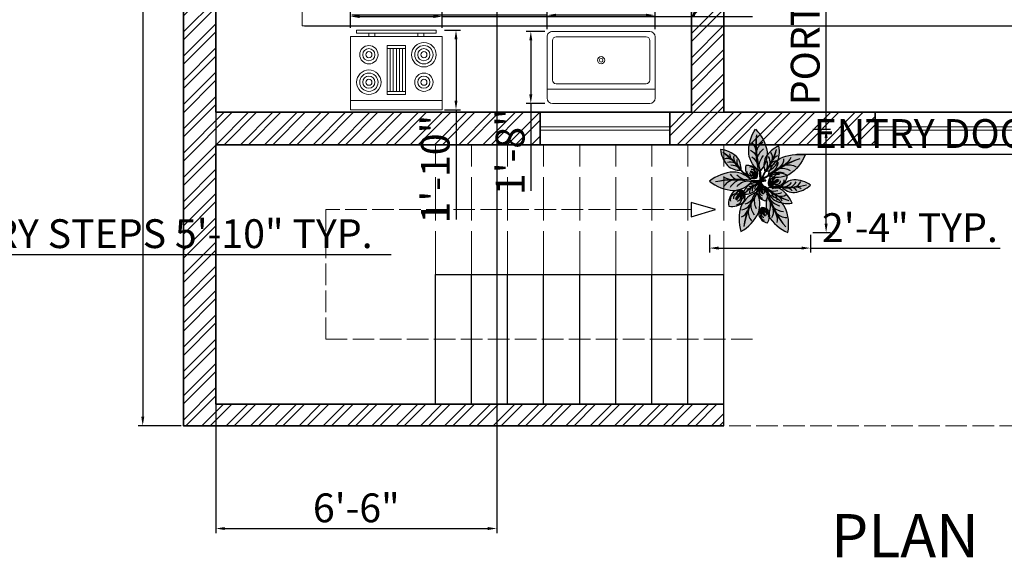
# Model space of a CAD drawing. Units: inches. Extents: x 3595 to 4516, y 2363 to 2965.
# Tile 6 of 12: x 4036 to 4309, y 2363 to 2512. Entities that reach past the tile are written whole.
import ezdxf

# ---------------------------------------------------------------- set-up
doc = ezdxf.new("R2010")
doc.units = ezdxf.units.IN
doc.linetypes.add('ACAD_ISO02W100', pattern=[15, 12, -3])
for name, color, linetype, lineweight in [('A-ANNO-DIMS', 2, 'Continuous', 18), ('A-ANNO-TEXT', 7, 'Continuous', 25), ('A-EQPM', 8, 'Continuous', 18), ('A-FLOR-CASE', 9, 'Continuous', 18), ('A-FLOR-FIXT', 8, 'Continuous', 18), ('A-FLOR-OTLN', 7, 'ACAD_ISO02W100', 18), ('A-FLOR-STRS', 7, 'Continuous', 25), ('A-FLOR-STRS-OVHD', 7, 'ACAD_ISO02W100', 18), ('A-GLAZ', 4, 'Continuous', 18), ('A-WALL', 7, 'Continuous', 35), ('L-PLNT', 3, 'Continuous', 13)]:
    doc.layers.add(name, color=color, linetype=linetype, lineweight=lineweight)
doc.layers.add('A-WALL-PATT', color=251, linetype='Continuous', lineweight=13, true_color=0x636466)
doc.layers.add('MESA', color=7, linetype='Continuous')
doc.styles.get("Standard").update_dxf_attribs({"font": 'arial.ttf'})
doc.dimstyles.new('ISO-25', dxfattribs={"dimtxt": 8, "dimasz": 2.5, "dimexe": 1.25, "dimexo": 0.625, "dimtad": 1, "dimdec": 1, "dimlunit": 3, "dimtxsty": 'Standard', "dimcen": 2.5, "dimadec": 0, "dimazin": 0, "dimtfac": 1, "dimtdec": 1, "dimtmove": 0, "dimatfit": 3, "dimfxl": 1, "dimarcsym": 0})

# ---------------------------------------------------------------- blocks, each defined once
blk = doc.blocks.new('*D6')
at = {"layer": 'A-ANNO-DIMS', "color": 0, "lineweight": -2, "transparency": 16777216}
for p, q in [((4080.62, 2903.04), (4068.71, 2903.04)), ((4069.96, 2900.54), (4069.96, 2401.54)), ((4080.62, 2399.04), (4068.71, 2399.04))]:
    blk.add_line(p, q, dxfattribs=at)
at = {"layer": 'A-ANNO-DIMS', "color": 0, "transparency": 16777216}
for points in [[(4069.55, 2900.54), (4070.38, 2900.54), (4069.96, 2903.04)], [(4069.55, 2401.54), (4070.38, 2401.54), (4069.96, 2399.04)]]:
    blk.add_solid(points, dxfattribs=at)
at = {"layer": 'Defpoints', "color": 0, "transparency": 16777216}
for p in [(4081.24, 2903.04), (4069.96, 2399.04), (4081.24, 2399.04)]:
    blk.add_point(p, dxfattribs=at)
at = {"layer": 'A-ANNO-DIMS', "color": 0, "transparency": 16777216, "insert": (4065.32, 2651.04), "char_height": 8, "attachment_point": 5, "rotation": 90}
blk.add_mtext("42'", dxfattribs=at)
blk = doc.blocks.new('folha Ant')
at = {"layer": 'MESA', "ltscale": 0.8}
h = blk.add_hatch(color=256, dxfattribs=at)
h.dxf.hatch_style = 1
h.set_gradient(color1=(179, 116, 77), color2=(114, 74, 49), one_color=1, tint=0.32, name='CURVED')
h.paths.add_polyline_path([(0.05, -0.0003), (0.0485, 0.0057, 0.033108), (0, 0, 0.809082), (0.002, -0.006, -0.032777)])
h.paths.add_polyline_path([(0.0973, 0.0049, 0.033108), (0.0485, 0.0057), (0.05, -0.0003, -0.032777), (0.0983, -0.001), (0.0953, 0.0026)])
h = blk.add_hatch(color=256, dxfattribs=at)
h.dxf.hatch_style = 1
h.set_gradient(color1=(103, 159, 96), color2=(52, 80, 48), one_color=1, tint=0.25)
h.paths.add_polyline_path([(0.3533, 0.0075, -0.09675), (0.0989, 0.0067, 0.007527), (0.0953, 0.0026, 0.014292), (0.1023, -0.0053, 0.086654)])
h = blk.add_hatch(color=256, dxfattribs=at)
h.dxf.hatch_style = 1
h.set_gradient(color1=(103, 159, 96), color2=(179, 207, 175), one_color=1, tint=0.75, name='INVCURVED')
h.paths.add_polyline_path([(0.2266, 0.0676, 0.199512), (0.0989, 0.0067, 0.09675), (0.3533, 0.0075, -0.086654), (0.1023, -0.0053, 0.192489), (0.2266, -0.0624, 0.158608), (0.3953, 0.0026, 0.158608)])
blk.add_lwpolyline([(0.0983, -0.001), (0.0953, 0.0026), (0.0973, 0.0049, 0.066288), (0, 0, 0.809082), (0.002, -0.006, -0.065625)], format="xyb", close=True, dxfattribs=at)
for centre, radius, start, end in [((0.2359, -0.1164), 0.1842, 92.91214, 139.76953), ((0.2359, 0.1215), 0.1842, 220.23047, 267.08786), ((0.2242, 0.6583), 0.6635, 259.11898, 281.22354), ((0.1912, 0.7199), 0.7306, 263.00966, 282.81986), ((0.1144, 0.1192), 0.1187, 277.64114, 318.48201), ((0.1515, 0.1013), 0.1129, 290.56342, 330.45391), ((0.211, -0.2242), 0.2922, 50.90546, 86.95539), ((0.211, 0.2293), 0.2922, 273.04461, 309.09454), ((0.2123, 0.0879), 0.0955, 283.00127, 333.19107), ((0.1127, -0.1239), 0.1214, 41.75279, 70.10606), ((0.1853, -0.0821), 0.0727, 27.73756, 79.23475), ((0.2381, -0.0995), 0.0902, 48.80268, 88.01103)]:
    blk.add_arc(centre, radius, start, end, dxfattribs=at)
blk = doc.blocks.new('folha A')
at = {"layer": 'MESA', "ltscale": 0.8}
h = blk.add_hatch(color=256, dxfattribs=at)
h.dxf.hatch_style = 1
h.set_gradient(color1=(237, 238, 238), one_color=1, tint=1)
h.paths.add_polyline_path([(0.15, 0, 0.256909), (0.0543, 0.05, 0.240303), (0.0028, 0.0075, -0.358381), (0.0489, 0.0306, 0.270233), (0, 0, -0.348977), (0.0363, 0.0149, 0.25095), (0.0039, 0, -0.245389), (0.0298, 0.008, 0.153246), (0.0082, 0, 0.15184), (0.0296, -0.008, 0.001374), (0.0298, -0.008, -0.245389), (0.0039, 0, 0.25095), (0.0363, -0.0149, -0.348977), (0, 0, 0.270233), (0.0489, -0.0306, -0.358381), (0.0028, -0.0075, 0.240303), (0.0543, -0.05, 0.256909)])
edge = h.paths.add_edge_path(flags=16)
edge.add_arc((0.0098, 0.0552), 0.0552, 269.91603, 271.41539, ccw=False)
edge.add_arc((0.011, -0.0487), 0.0487, 89.81625, 91.51517, ccw=False)
edge.add_arc((0.0098, 0.0552), 0.0552, 271.41539, 288.97446)
edge.add_spline(control_points=[(0.0278, 0.003), (0.0281, 0.003), (0.03, 0.0028), (0.032, 0.0025), (0.0337, 0.0022)], knot_values=[0.247151, 0.247151, 0.247151, 0.247151, 0.247786, 0.253074, 0.253074, 0.253074, 0.253074], degree=3, periodic=0)
edge.add_spline(control_points=[(0.0337, 0.0022), (0.0349, 0.0021), (0.0361, 0.0019), (0.0372, 0.0017)], knot_values=[0.243636, 0.243636, 0.243636, 0.243636, 0.247151, 0.247151, 0.247151, 0.247151], degree=3, periodic=0)
edge.add_spline(control_points=[(0.0372, 0.0017), (0.0385, 0.0015), (0.0405, 0.0013), (0.0424, 0.0011), (0.0431, 0.0011)], knot_values=[0.23773, 0.23773, 0.23773, 0.23773, 0.241748, 0.243636, 0.243636, 0.243636, 0.243636], degree=3, periodic=0)
edge.add_spline(control_points=[(0.0431, 0.0011), (0.044, 0.001), (0.045, 0.001), (0.0459, 0.001)], knot_values=[0.234818, 0.234818, 0.234818, 0.234818, 0.23773, 0.23773, 0.23773, 0.23773], degree=3, periodic=0)
edge.add_spline(control_points=[(0.0459, 0.001), (0.0472, 0.0009), (0.0485, 0.0009), (0.0498, 0.0009)], knot_values=[0.230931, 0.230931, 0.230931, 0.230931, 0.234818, 0.234818, 0.234818, 0.234818], degree=3, periodic=0)
edge.add_spline(control_points=[(0.0498, 0.0009), (0.0513, 0.0009), (0.0528, 0.0009), (0.0543, 0.0009)], knot_values=[0.226471, 0.226471, 0.226471, 0.226471, 0.230931, 0.230931, 0.230931, 0.230931], degree=3, periodic=0)
edge.add_spline(control_points=[(0.0543, 0.0009), (0.0547, 0.0009), (0.0564, 0.001), (0.0581, 0.001), (0.0594, 0.0011)], knot_values=[0.221526, 0.221526, 0.221526, 0.221526, 0.222579, 0.226471, 0.226471, 0.226471, 0.226471], degree=3, periodic=0)
edge.add_spline(control_points=[(0.0594, 0.0011), (0.0609, 0.0012), (0.0623, 0.0014), (0.0637, 0.0017)], knot_values=[0.217168, 0.217168, 0.217168, 0.217168, 0.221526, 0.221526, 0.221526, 0.221526], degree=3, periodic=0)
edge.add_spline(control_points=[(0.0637, 0.0017), (0.0648, 0.002), (0.066, 0.0024), (0.0672, 0.0029), (0.0674, 0.003)], knot_values=[0.213164, 0.213164, 0.213164, 0.213164, 0.216463, 0.217168, 0.217168, 0.217168, 0.217168], degree=3, periodic=0)
edge.add_spline(control_points=[(0.0674, 0.003), (0.0685, 0.0035), (0.07, 0.0044), (0.0718, 0.0051), (0.0724, 0.0052)], knot_values=[0.207777, 0.207777, 0.207777, 0.207777, 0.211372, 0.213164, 0.213164, 0.213164, 0.213164], degree=3, periodic=0)
edge.add_spline(control_points=[(0.0724, 0.0052), (0.0729, 0.0053), (0.0744, 0.0054), (0.0757, 0.0044), (0.0762, 0.0036)], knot_values=[0.203445, 0.203445, 0.203445, 0.203445, 0.204995, 0.207777, 0.207777, 0.207777, 0.207777], degree=3, periodic=0)
edge.add_spline(control_points=[(0.0762, 0.0036), (0.0763, 0.0036), (0.0768, 0.0026), (0.0767, 0.0012), (0.0763, 0), (0.0763, -0.0001)], knot_values=[0.199694, 0.199694, 0.199694, 0.199694, 0.199863, 0.203137, 0.203445, 0.203445, 0.203445, 0.203445], degree=3, periodic=0)
edge.add_spline(control_points=[(0.0763, -0.0001), (0.0761, -0.0008), (0.0757, -0.0017), (0.075, -0.0024), (0.0748, -0.0026)], knot_values=[0.196756, 0.196756, 0.196756, 0.196756, 0.198903, 0.199694, 0.199694, 0.199694, 0.199694], degree=3, periodic=0)
edge.add_spline(control_points=[(0.0748, -0.0026), (0.0743, -0.0031), (0.0734, -0.0037), (0.0725, -0.0042), (0.0722, -0.0043)], knot_values=[0.193643, 0.193643, 0.193643, 0.193643, 0.195869, 0.196756, 0.196756, 0.196756, 0.196756], degree=3, periodic=0)
edge.add_spline(control_points=[(0.0722, -0.0043), (0.0708, -0.0049), (0.0694, -0.0052), (0.0678, -0.0054)], knot_values=[0.189135, 0.189135, 0.189135, 0.189135, 0.193643, 0.193643, 0.193643, 0.193643], degree=3, periodic=0)
edge.add_spline(control_points=[(0.0678, -0.0054), (0.0677, -0.0054), (0.0667, -0.0056), (0.0657, -0.0057), (0.0648, -0.0058)], knot_values=[0.186092, 0.186092, 0.186092, 0.186092, 0.186502, 0.189135, 0.189135, 0.189135, 0.189135], degree=3, periodic=0)
edge.add_spline(control_points=[(0.0648, -0.0058), (0.0635, -0.0059), (0.0621, -0.006), (0.0608, -0.0061)], knot_values=[0.182083, 0.182083, 0.182083, 0.182083, 0.186092, 0.186092, 0.186092, 0.186092], degree=3, periodic=0)
edge.add_spline(control_points=[(0.0608, -0.0061), (0.0596, -0.0062), (0.0584, -0.0062), (0.0571, -0.0062)], knot_values=[0.178391, 0.178391, 0.178391, 0.178391, 0.182083, 0.182083, 0.182083, 0.182083], degree=3, periodic=0)
edge.add_spline(control_points=[(0.0571, -0.0062), (0.0568, -0.0062), (0.0555, -0.0063), (0.0543, -0.0063), (0.0534, -0.0063)], knot_values=[0.17468, 0.17468, 0.17468, 0.17468, 0.175797, 0.178391, 0.178391, 0.178391, 0.178391], degree=3, periodic=0)
edge.add_spline(control_points=[(0.0534, -0.0063), (0.0525, -0.0063), (0.0516, -0.0063), (0.0506, -0.0063)], knot_values=[0.171864, 0.171864, 0.171864, 0.171864, 0.17468, 0.17468, 0.17468, 0.17468], degree=3, periodic=0)
edge.add_spline(control_points=[(0.0506, -0.0063), (0.0494, -0.0063), (0.0482, -0.0063), (0.047, -0.0062)], knot_values=[0.16826, 0.16826, 0.16826, 0.16826, 0.171864, 0.171864, 0.171864, 0.171864], degree=3, periodic=0)
edge.add_spline(control_points=[(0.047, -0.0062), (0.0453, -0.0061), (0.0434, -0.006), (0.0414, -0.0057), (0.0411, -0.0057)], knot_values=[0.162342, 0.162342, 0.162342, 0.162342, 0.167388, 0.16826, 0.16826, 0.16826, 0.16826], degree=3, periodic=0)
edge.add_spline(control_points=[(0.0411, -0.0057), (0.0399, -0.0055), (0.0386, -0.0053), (0.0374, -0.005)], knot_values=[0.158654, 0.158654, 0.158654, 0.158654, 0.162342, 0.162342, 0.162342, 0.162342], degree=3, periodic=0)
edge.add_spline(control_points=[(0.0374, -0.005), (0.0365, -0.0049), (0.0357, -0.0047), (0.0348, -0.0045)], knot_values=[0.156033, 0.156033, 0.156033, 0.156033, 0.158654, 0.158654, 0.158654, 0.158654], degree=3, periodic=0)
edge.add_spline(control_points=[(0.0348, -0.0045), (0.0335, -0.0043), (0.0317, -0.004), (0.03, -0.0037), (0.0295, -0.0036)], knot_values=[0.15048, 0.15048, 0.15048, 0.15048, 0.154549, 0.156033, 0.156033, 0.156033, 0.156033], degree=3, periodic=0)
edge.add_arc((0.011, -0.0487), 0.0487, 67.70537, 89.81625)
h = blk.add_hatch(color=256, dxfattribs=at)
h.dxf.hatch_style = 1
h.set_gradient(color1=(117, 211, 105), one_color=1, tint=1)
h.paths.add_polyline_path([(0.0489, 0.0306, 0.358381), (0.0028, 0.0075, 0.02724), (0, 0, -0.270233)])
h.paths.add_polyline_path([(0.0039, 0, -0.25095), (0.0363, 0.0149, 0.348977), (0, 0, 0.348977), (0.0363, -0.0149, -0.25095)])
h.paths.add_polyline_path([(0.0298, 0.008, 0.245389), (0.0039, 0, 0.245389), (0.0298, -0.008, -0.153246), (0.0082, 0, -0.153246)], flags=17)
h.paths.add_polyline_path([(0, 0, 0.02724), (0.0028, -0.0075, 0.358381), (0.0489, -0.0306, -0.270233)])
h = blk.add_hatch(color=256, dxfattribs=at)
h.dxf.hatch_style = 1
h.set_gradient(color1=(68, 182, 53), color2=(121, 213, 109), one_color=1, tint=0.63, name='CYLINDER')
edge = h.paths.add_edge_path()
edge.add_spline(control_points=[(0.0722, -0.0043), (0.0725, -0.0042), (0.0734, -0.0037), (0.0743, -0.0031), (0.0748, -0.0026)], knot_values=[0.193643, 0.193643, 0.193643, 0.193643, 0.194531, 0.196756, 0.196756, 0.196756, 0.196756], degree=3, periodic=0)
edge.add_spline(control_points=[(0.0748, -0.0026), (0.075, -0.0024), (0.0757, -0.0017), (0.0761, -0.0008), (0.0763, -0.0001)], knot_values=[0.196756, 0.196756, 0.196756, 0.196756, 0.197548, 0.199694, 0.199694, 0.199694, 0.199694], degree=3, periodic=0)
edge.add_spline(control_points=[(0.0763, -0.0001), (0.0763, 0), (0.0767, 0.0012), (0.0768, 0.0026), (0.0763, 0.0036), (0.0762, 0.0036)], knot_values=[0.199694, 0.199694, 0.199694, 0.199694, 0.200002, 0.203276, 0.203445, 0.203445, 0.203445, 0.203445], degree=3, periodic=0)
edge.add_spline(control_points=[(0.0762, 0.0036), (0.0757, 0.0044), (0.0744, 0.0054), (0.0729, 0.0053), (0.0724, 0.0052)], knot_values=[0.203445, 0.203445, 0.203445, 0.203445, 0.206228, 0.207777, 0.207777, 0.207777, 0.207777], degree=3, periodic=0)
edge.add_spline(control_points=[(0.0724, 0.0052), (0.0718, 0.0051), (0.07, 0.0044), (0.0685, 0.0035), (0.0674, 0.003)], knot_values=[0.207777, 0.207777, 0.207777, 0.207777, 0.20957, 0.213164, 0.213164, 0.213164, 0.213164], degree=3, periodic=0)
edge.add_spline(control_points=[(0.0674, 0.003), (0.0672, 0.0029), (0.066, 0.0024), (0.0648, 0.002), (0.0637, 0.0017)], knot_values=[0.213164, 0.213164, 0.213164, 0.213164, 0.213868, 0.217168, 0.217168, 0.217168, 0.217168], degree=3, periodic=0)
edge.add_spline(control_points=[(0.0637, 0.0017), (0.0623, 0.0014), (0.0609, 0.0012), (0.0594, 0.0011)], knot_values=[0.217168, 0.217168, 0.217168, 0.217168, 0.221526, 0.221526, 0.221526, 0.221526], degree=3, periodic=0)
edge.add_spline(control_points=[(0.0594, 0.0011), (0.0581, 0.001), (0.0564, 0.001), (0.0547, 0.0009), (0.0543, 0.0009)], knot_values=[0.221526, 0.221526, 0.221526, 0.221526, 0.225418, 0.226471, 0.226471, 0.226471, 0.226471], degree=3, periodic=0)
edge.add_spline(control_points=[(0.0543, 0.0009), (0.0528, 0.0009), (0.0513, 0.0009), (0.0498, 0.0009)], knot_values=[0.226471, 0.226471, 0.226471, 0.226471, 0.230931, 0.230931, 0.230931, 0.230931], degree=3, periodic=0)
edge.add_spline(control_points=[(0.0498, 0.0009), (0.0485, 0.0009), (0.0472, 0.0009), (0.0459, 0.001)], knot_values=[0.230931, 0.230931, 0.230931, 0.230931, 0.234818, 0.234818, 0.234818, 0.234818], degree=3, periodic=0)
edge.add_spline(control_points=[(0.0459, 0.001), (0.045, 0.001), (0.044, 0.001), (0.0431, 0.0011)], knot_values=[0.234818, 0.234818, 0.234818, 0.234818, 0.23773, 0.23773, 0.23773, 0.23773], degree=3, periodic=0)
edge.add_spline(control_points=[(0.0431, 0.0011), (0.0424, 0.0011), (0.0405, 0.0013), (0.0385, 0.0015), (0.0372, 0.0017)], knot_values=[0.23773, 0.23773, 0.23773, 0.23773, 0.239619, 0.243636, 0.243636, 0.243636, 0.243636], degree=3, periodic=0)
edge.add_spline(control_points=[(0.0372, 0.0017), (0.0361, 0.0019), (0.0349, 0.0021), (0.0337, 0.0022)], knot_values=[0.243636, 0.243636, 0.243636, 0.243636, 0.247151, 0.247151, 0.247151, 0.247151], degree=3, periodic=0)
edge.add_spline(control_points=[(0.0337, 0.0022), (0.032, 0.0025), (0.03, 0.0028), (0.0281, 0.003), (0.0278, 0.003)], knot_values=[0.247151, 0.247151, 0.247151, 0.247151, 0.25244, 0.253074, 0.253074, 0.253074, 0.253074], degree=3, periodic=0)
edge.add_arc((0.011, 0.0487), 0.0487, 271.51517, 290.22735, ccw=False)
edge.add_arc((0.011, -0.0487), 0.0487, 67.70537, 88.48483, ccw=False)
edge.add_spline(control_points=[(0.0295, -0.0036), (0.03, -0.0037), (0.0317, -0.004), (0.0335, -0.0043), (0.0348, -0.0045)], knot_values=[0.15048, 0.15048, 0.15048, 0.15048, 0.151964, 0.156033, 0.156033, 0.156033, 0.156033], degree=3, periodic=0)
edge.add_spline(control_points=[(0.0348, -0.0045), (0.0357, -0.0047), (0.0365, -0.0049), (0.0374, -0.005)], knot_values=[0.156033, 0.156033, 0.156033, 0.156033, 0.158654, 0.158654, 0.158654, 0.158654], degree=3, periodic=0)
edge.add_spline(control_points=[(0.0374, -0.005), (0.0386, -0.0053), (0.0399, -0.0055), (0.0411, -0.0057)], knot_values=[0.158654, 0.158654, 0.158654, 0.158654, 0.162342, 0.162342, 0.162342, 0.162342], degree=3, periodic=0)
edge.add_spline(control_points=[(0.0411, -0.0057), (0.0414, -0.0057), (0.0434, -0.006), (0.0453, -0.0061), (0.047, -0.0062)], knot_values=[0.162342, 0.162342, 0.162342, 0.162342, 0.163214, 0.16826, 0.16826, 0.16826, 0.16826], degree=3, periodic=0)
edge.add_spline(control_points=[(0.047, -0.0062), (0.0482, -0.0063), (0.0494, -0.0063), (0.0506, -0.0063)], knot_values=[0.16826, 0.16826, 0.16826, 0.16826, 0.171864, 0.171864, 0.171864, 0.171864], degree=3, periodic=0)
edge.add_spline(control_points=[(0.0506, -0.0063), (0.0516, -0.0063), (0.0525, -0.0063), (0.0534, -0.0063)], knot_values=[0.171864, 0.171864, 0.171864, 0.171864, 0.17468, 0.17468, 0.17468, 0.17468], degree=3, periodic=0)
edge.add_spline(control_points=[(0.0534, -0.0063), (0.0543, -0.0063), (0.0555, -0.0063), (0.0568, -0.0062), (0.0571, -0.0062)], knot_values=[0.17468, 0.17468, 0.17468, 0.17468, 0.177274, 0.178391, 0.178391, 0.178391, 0.178391], degree=3, periodic=0)
edge.add_spline(control_points=[(0.0571, -0.0062), (0.0584, -0.0062), (0.0596, -0.0062), (0.0608, -0.0061)], knot_values=[0.178391, 0.178391, 0.178391, 0.178391, 0.182083, 0.182083, 0.182083, 0.182083], degree=3, periodic=0)
edge.add_spline(control_points=[(0.0608, -0.0061), (0.0621, -0.006), (0.0635, -0.0059), (0.0648, -0.0058)], knot_values=[0.182083, 0.182083, 0.182083, 0.182083, 0.186092, 0.186092, 0.186092, 0.186092], degree=3, periodic=0)
edge.add_spline(control_points=[(0.0648, -0.0058), (0.0657, -0.0057), (0.0667, -0.0056), (0.0677, -0.0054), (0.0678, -0.0054)], knot_values=[0.186092, 0.186092, 0.186092, 0.186092, 0.188726, 0.189135, 0.189135, 0.189135, 0.189135], degree=3, periodic=0)
edge.add_spline(control_points=[(0.0678, -0.0054), (0.0694, -0.0052), (0.0708, -0.0049), (0.0722, -0.0043)], knot_values=[0.189135, 0.189135, 0.189135, 0.189135, 0.193643, 0.193643, 0.193643, 0.193643], degree=3, periodic=0)
for p, q in [((0.0299, -0.0008), (0.0236, 0.0003)), ((0.0324, 0.0004), (0.0358, 0.0051)), ((0.0367, 0.001), (0.0414, 0.0073)), ((0.0435, -0.0027), (0.0427, 0.0041)), ((0.0455, -0.0007), (0.0466, 0.0032)), ((0.0507, -0.0021), (0.0477, 0.0086)), ((0.0545, -0.0006), (0.0538, 0.005)), ((0.0604, -0.0013), (0.0571, 0.0065)), ((0.0637, -0.0003), (0.0638, 0.0057)), ((0.0674, 0.0003), (0.0674, 0.0088)), ((0.071, 0.0011), (0.0736, 0.0087)), ((0.0744, 0.0005), (0.0836, -0.0024)), ((0.0745, 0.0023), (0.0809, 0.0072)), ((0.0331, -0.0017), (0.0356, -0.0058)), ((0.0359, -0.0021), (0.0384, -0.0071)), ((0.04, -0.0018), (0.0423, -0.0098)), ((0.0474, -0.0047), (0.0459, -0.0105)), ((0.0512, -0.005), (0.0493, -0.009)), ((0.0546, -0.0037), (0.0519, -0.0097)), ((0.0571, -0.0045), (0.0573, -0.0126)), ((0.0629, -0.0036), (0.0579, -0.0096)), ((0.0649, -0.0044), (0.0646, -0.0097)), ((0.0679, -0.003), (0.0676, -0.0121)), ((0.0718, -0.0029), (0.0733, -0.0082)), ((0.0731, -0.0013), (0.0781, -0.005))]:
    blk.add_line(p, q, dxfattribs=at)
for centre, radius, start, end in [((0.0702, -0.0218), 0.0735, 102.48764, 162.77768), ((0.0507, -0.0267), 0.0573, 91.76636, 152.2545), ((0.0275, -0.0154), 0.0315, 73.89832, 150.84957), ((0.0399, -0.009), 0.0406, 77.14264, 158.36501), ((0.034, -0.0228), 0.0378, 86.58524, 142.93515), ((0.0245, -0.0208), 0.0293, 79.57473, 134.72404), ((0.0317, -0.0305), 0.0385, 92.86525, 127.71548), ((0.0067, 0.0482), 0.0483, 273.5313, 328.711), ((0.0098, 0.0552), 0.0552, 269.91603, 311.56133), ((0.011, -0.0487), 0.0487, 43.37027, 91.51517), ((0.0655, -0.0023), 0.025, 51.97118, 139.68499), ((0.0788, 0.0012), 0.0378, 48.94459, 144.53335), ((0.0567, -0.062), 0.112, 33.59498, 91.22784), ((0.0507, 0.0267), 0.0573, 207.7455, 268.23364), ((0.0275, 0.0154), 0.0315, 209.15043, 286.10168), ((0.0702, 0.0218), 0.0735, 197.22232, 257.51236), ((0.0399, 0.009), 0.0406, 201.63499, 282.85736), ((0.034, 0.0228), 0.0378, 217.06485, 273.41476), ((0.0245, 0.0208), 0.0293, 225.27596, 280.42527), ((0.0317, 0.0305), 0.0385, 232.28452, 267.13475), ((0.0067, -0.0482), 0.0483, 31.289, 86.4687), ((0.0676, -0.0011), 0.0254, 213.67702, 332.84146), ((0.0804, 0.0017), 0.0409, 217.4348, 331.73221), ((0.0567, 0.062), 0.112, 268.77216, 326.40502)]:
    blk.add_arc(centre, radius, start, end, dxfattribs=at)
blk.add_open_spline([(0.0295, -0.0036), (0.03, -0.0037), (0.0339, -0.0043), (0.0429, -0.0064), (0.0552, -0.0064), (0.0655, -0.0059), (0.0723, -0.0047), (0.0754, -0.0023), (0.0766, 0.0004), (0.0769, 0.0036), (0.0738, 0.0058), (0.0702, 0.0046), (0.0648, 0.0013), (0.0544, 0.0009), (0.0416, 0.0008), (0.0325, 0.0025), (0.0281, 0.003), (0.0278, 0.003)], degree=3, knots=[0.1504802, 0.1504802, 0.1504802, 0.1504802, 0.1519644, 0.163214, 0.177274, 0.1887256, 0.1945307, 0.1975476, 0.2000024, 0.2032763, 0.2062279, 0.2095699, 0.2138685, 0.2254176, 0.2396186, 0.2524399, 0.2530743, 0.2530743, 0.2530743, 0.2530743], dxfattribs=at)
blk = doc.blocks.new('Anturio Completa')
at = {"layer": 'MESA', "xscale": -1}
for p, rotation in [((0.0382, -0.3934), 275.9103487005753), ((0.0047, -0.3743), 209.3422747969654)]:
    blk.add_blockref('folha Ant', p, dxfattribs=dict(at, rotation=rotation))
at = {"layer": 'MESA'}
for name, p, xscale, yscale, zscale, rotation in [('folha Ant', (-0.0545, -0.3355), 0.6875195991113106, 0.6875195991113106, 0.6875195991113106, 134.6123703789177), ('folha Ant', (0.0396, -0.3604), 0.6875195991112988, 0.6875195991112988, 0.6875195991112988, 62.02852832027476), ('folha A', (0.0091, -0.3436), 0.7678141644548924, 0.7678141644548924, 0.7678141644548924, 132.2423739965673), ('folha Ant', (0.06, -0.3566), 0.4588451896756128, 0.4588451896756128, 0.4588451896756128, 214.0760858842101), ('folha Ant', (0.0225, -0.3869), 0.6875195991113232, 0.6875195991113232, 0.6875195991113232, 329.7037252995857), ('folha A', (0.0322, -0.3992), 0.7678141644548587, 0.7678141644548587, 0.7678141644548587, 290.0444626994612), ('folha Ant', (0.1178, -0.4144), 0.6875195991112375, 0.6875195991112375, 0.6875195991112375, 3.732606609119443), ('folha A', (0.0446, -0.5537), 0.7678141644548587, 0.7678141644548587, 0.7678141644548587, 290.0444626994612)]:
    blk.add_blockref(name, p, dxfattribs=dict(at, xscale=xscale, yscale=yscale, zscale=zscale, rotation=rotation))
for name, p, rotation in [('folha Ant', (0.0722, -0.3656), 180), ('folha Ant', (0.0428, -0.3558), 248.0349850699403), ('folha A', (0.0917, -0.3951), 27.20904127110871), ('folha A', (-0.0806, -0.4387), 224.8255080541778), ('folha Ant', (0.0423, -0.3813), 297.7195320534174)]:
    blk.add_blockref(name, p, dxfattribs=dict(at, rotation=rotation))
blk = doc.blocks.new('Range-Oven - 30 in top')
for p, q in [((0, -3), (30, -3)), ((12, -6), (18, -6)), ((13, -20), (13, -6)), ((14, -6), (14, -20)), ((15, -20), (15, -6)), ((16, -6), (16, -20)), ((17, -20), (17, -6)), ((18, -20), (12, -20)), ((6, -24), (6, -25)), ((8, -25), (8, -24)), ((22, -25), (22, -24)), ((24, -24), (24, -25))]:
    blk.add_line(p, q)
for points in [[(0, -24), (0, 0), (30, 0), (30, -24)], [(12, -21), (12, -5), (18, -5), (18, -21)], [(2, -26), (2, -25), (28, -25), (28, -26)]]:
    blk.add_lwpolyline(points, close=True)
for centre, radius in [((6, -9), 4), ((6, -9), 3), ((24, -9), 3), ((6, -9), 2), ((6, -9), 1), ((24, -9), 2), ((24, -9), 1), ((6, -18), 3), ((6, -18), 2), ((24, -18), 4), ((24, -18), 3), ((24, -18), 2), ((6, -18), 1), ((24, -18), 1)]:
    blk.add_circle(centre, radius)
blk = doc.blocks.new('Sink-single - 30 in top')
blk.add_line((-15, -3.999996), (15, -3.999996))
for points in [[(-13.5, 0), (13.5, 0)], [(-15, -18.499996), (-15, -1.5)], [(15, -1.5), (15, -18.499996)], [(-13.5, -17.499996), (-13.5, -6.499996)], [(-12.5, -5.499996), (12.5, -5.499996)], [(13.5, -6.499996), (13.5, -17.499996)], [(12.5, -18.499996), (-12.5, -18.499996)], [(13.5, -19.999996), (-13.5, -19.999996)]]:
    blk.add_lwpolyline(points)
for radius in [1, 0.5]:
    blk.add_circle((0, -11.999996), radius)
for centre, radius, start, end in [((-13.5, -1.5), 1.5, 90, 180), ((13.5, -1.5), 1.5, 0, 90), ((-12.5, -6.499996), 1, 90, 180), ((12.5, -6.499996), 1, 0, 90), ((-13.5, -18.499996), 1.5, 180, 270), ((-12.5, -17.499996), 1, 180, 270), ((12.5, -17.499996), 1, 270, 0), ((13.5, -18.499996), 1.5, 270, 0)]:
    blk.add_arc(centre, radius, start, end)
blk = doc.blocks.new('WIN-GLAZING-66IN')
for p, q in [((0, 1), (66, 1)), ((0, 0), (66, 0))]:
    blk.add_line(p, q)
blk = doc.blocks.new('WIN-GLAZING-36IN')
for p, q in [((0, 1), (36, 1)), ((0, 0), (36, 0))]:
    blk.add_line(p, q)
blk = doc.blocks.new('*D113')
at = {"layer": 'A-ANNO-DIMS', "color": 0, "lineweight": -2, "transparency": 16777216}
for p, q in [((4381.24, 2480.92), (4381.24, 2473.09)), ((4429.24, 2480.92), (4429.24, 2473.09)), ((4381.24, 2474.34), (4251.53, 2474.34)), ((4426.74, 2474.34), (4383.74, 2474.34))]:
    blk.add_line(p, q, dxfattribs=at)
at = {"layer": 'A-ANNO-DIMS', "color": 0, "transparency": 16777216}
for points in [[(4383.74, 2474.76), (4383.74, 2473.93), (4381.24, 2474.34)], [(4426.74, 2474.76), (4426.74, 2473.93), (4429.24, 2474.34)]]:
    blk.add_solid(points, dxfattribs=at)
at = {"layer": 'Defpoints', "color": 0, "transparency": 16777216}
for p in [(4381.24, 2481.54), (4429.24, 2481.54), (4381.24, 2474.34)]:
    blk.add_point(p, dxfattribs=at)
at = {"layer": 'A-ANNO-DIMS', "color": 0, "transparency": 16777216, "insert": (4315.14, 2479.11), "char_height": 8, "attachment_point": 5}
blk.add_mtext('ENTRY DOOR 4\'-0" TYP.', dxfattribs=at)
blk = doc.blocks.new('*D117')
at = {"layer": 'A-ANNO-DIMS', "color": 0, "lineweight": -2, "transparency": 16777216}
for p, q in [((3929.89, 2456.42), (3929.89, 2445.29)), ((3999.89, 2456.42), (3999.89, 2445.29)), ((3932.39, 2446.54), (3997.39, 2446.54)), ((3999.89, 2446.54), (4138.93, 2446.54))]:
    blk.add_line(p, q, dxfattribs=at)
at = {"layer": 'A-ANNO-DIMS', "color": 0, "transparency": 16777216}
for points in [[(3932.39, 2446.96), (3932.39, 2446.13), (3929.89, 2446.54)], [(3997.39, 2446.96), (3997.39, 2446.13), (3999.89, 2446.54)]]:
    blk.add_solid(points, dxfattribs=at)
at = {"layer": 'Defpoints', "color": 0, "transparency": 16777216}
for p in [(3929.89, 2457.04), (3999.89, 2457.04), (3999.89, 2446.54)]:
    blk.add_point(p, dxfattribs=at)
at = {"layer": 'A-ANNO-DIMS', "color": 0, "transparency": 16777216, "insert": (4070.66, 2451.31), "char_height": 8, "attachment_point": 5}
blk.add_mtext('ENTRY STEPS 5\'-10" TYP.', dxfattribs=at)
blk = doc.blocks.new('*D135')
at = {"layer": 'A-ANNO-DIMS', "color": 0, "lineweight": -2, "transparency": 16777216}
for p, q in [((4127.63, 2509.45), (4127.63, 2513.89)), ((4130.13, 2512.64), (4150.59, 2512.64)), ((4153.09, 2509.45), (4153.09, 2513.89)), ((4153.09, 2512.64), (4239.18, 2512.64))]:
    blk.add_line(p, q, dxfattribs=at)
at = {"layer": 'A-ANNO-DIMS', "color": 0, "transparency": 16777216}
for points in [[(4130.13, 2513.06), (4130.13, 2512.22), (4127.63, 2512.64)], [(4150.59, 2513.06), (4150.59, 2512.22), (4153.09, 2512.64)]]:
    blk.add_solid(points, dxfattribs=at)
at = {"layer": 'Defpoints', "color": 0, "transparency": 16777216}
for p in [(4153.09, 2512.64), (4127.63, 2508.82), (4153.09, 2508.82)]:
    blk.add_point(p, dxfattribs=at)
at = {"layer": 'A-ANNO-DIMS', "color": 0, "transparency": 16777216, "insert": (4197.38, 2517.4), "char_height": 8, "attachment_point": 5}
blk.add_mtext('RANGE 2\'-1 1/2"', dxfattribs=at)
blk = doc.blocks.new('*D136')
at = {"layer": 'A-ANNO-DIMS', "color": 0, "lineweight": -2, "transparency": 16777216}
for p, q in [((4153.71, 2508.82), (4158.16, 2508.82)), ((4156.91, 2506.32), (4156.91, 2489.26)), ((4153.71, 2486.76), (4158.16, 2486.76)), ((4156.91, 2486.76), (4156.91, 2456.28))]:
    blk.add_line(p, q, dxfattribs=at)
at = {"layer": 'A-ANNO-DIMS', "color": 0, "transparency": 16777216}
for points in [[(4156.49, 2506.32), (4157.32, 2506.32), (4156.91, 2508.82)], [(4156.49, 2489.26), (4157.32, 2489.26), (4156.91, 2486.76)]]:
    blk.add_solid(points, dxfattribs=at)
at = {"layer": 'Defpoints', "color": 0, "transparency": 16777216}
for p in [(4153.09, 2508.82), (4153.09, 2486.76), (4156.91, 2486.76)]:
    blk.add_point(p, dxfattribs=at)
at = {"layer": 'A-ANNO-DIMS', "color": 0, "transparency": 16777216, "insert": (4152.2, 2470.27), "char_height": 8, "attachment_point": 5, "rotation": 90}
blk.add_mtext('1\'-10"', dxfattribs=at)
blk = doc.blocks.new('*D137')
at = {"layer": 'A-ANNO-DIMS', "color": 0, "lineweight": -2, "transparency": 16777216}
for p, q in [((4182.18, 2512.99), (4128.01, 2512.99)), ((4182.18, 2509.12), (4182.18, 2514.24)), ((4209.68, 2512.99), (4184.68, 2512.99)), ((4212.18, 2509.12), (4212.18, 2514.24))]:
    blk.add_line(p, q, dxfattribs=at)
at = {"layer": 'A-ANNO-DIMS', "color": 0, "transparency": 16777216}
for points in [[(4184.68, 2513.41), (4184.68, 2512.58), (4182.18, 2512.99)], [(4209.68, 2513.41), (4209.68, 2512.58), (4212.18, 2512.99)]]:
    blk.add_solid(points, dxfattribs=at)
at = {"layer": 'Defpoints', "color": 0, "transparency": 16777216}
for p in [(4182.18, 2512.99), (4182.18, 2508.49), (4212.18, 2508.49)]:
    blk.add_point(p, dxfattribs=at)
at = {"layer": 'A-ANNO-DIMS', "color": 0, "transparency": 16777216, "insert": (4153.84, 2517.75), "char_height": 8, "attachment_point": 5}
blk.add_mtext('SINK 2\'-6"', dxfattribs=at)
blk = doc.blocks.new('*D138')
at = {"layer": 'A-ANNO-DIMS', "color": 0, "lineweight": -2, "transparency": 16777216}
for p, q in [((4181.55, 2508.49), (4176.43, 2508.49)), ((4177.68, 2505.99), (4177.68, 2490.99)), ((4181.55, 2488.49), (4176.43, 2488.49)), ((4177.68, 2488.49), (4177.68, 2464.23))]:
    blk.add_line(p, q, dxfattribs=at)
at = {"layer": 'A-ANNO-DIMS', "color": 0, "transparency": 16777216}
for points in [[(4177.26, 2505.99), (4178.09, 2505.99), (4177.68, 2508.49)], [(4177.26, 2490.99), (4178.09, 2490.99), (4177.68, 2488.49)]]:
    blk.add_solid(points, dxfattribs=at)
at = {"layer": 'Defpoints', "color": 0, "transparency": 16777216}
for p in [(4182.18, 2508.49), (4177.68, 2488.49), (4182.18, 2488.49)]:
    blk.add_point(p, dxfattribs=at)
at = {"layer": 'A-ANNO-DIMS', "color": 0, "transparency": 16777216, "insert": (4172.97, 2475.11), "char_height": 8, "attachment_point": 5, "rotation": 90}
blk.add_mtext('1\'-8"', dxfattribs=at)
blk = doc.blocks.new('*D145')
at = {"layer": 'A-ANNO-DIMS', "color": 0, "lineweight": -2, "transparency": 16777216}
for p, q in [((4259.64, 2481.4), (4259.64, 2645.3)), ((4255.95, 2481.4), (4260.89, 2481.4)), ((4259.64, 2455.16), (4259.64, 2478.9)), ((4255.95, 2452.66), (4260.89, 2452.66))]:
    blk.add_line(p, q, dxfattribs=at)
at = {"layer": 'A-ANNO-DIMS', "color": 0, "transparency": 16777216}
for points in [[(4259.22, 2478.9), (4260.06, 2478.9), (4259.64, 2481.4)], [(4259.22, 2455.16), (4260.06, 2455.16), (4259.64, 2452.66)]]:
    blk.add_solid(points, dxfattribs=at)
at = {"layer": 'Defpoints', "color": 0, "transparency": 16777216}
for p in [(4255.33, 2481.4), (4259.64, 2481.4), (4255.33, 2452.66)]:
    blk.add_point(p, dxfattribs=at)
at = {"layer": 'A-ANNO-DIMS', "color": 0, "transparency": 16777216, "insert": (4254.87, 2564.6), "char_height": 8, "attachment_point": 5, "rotation": 90}
blk.add_mtext('PORTICO PLANT 2\'-4 1/2" TYP.', dxfattribs=at)
blk = doc.blocks.new('*D146')
at = {"layer": 'A-ANNO-DIMS', "color": 0, "lineweight": -2, "transparency": 16777216}
for p, q in [((4227.3, 2452.03), (4227.3, 2447.1)), ((4255.33, 2452.03), (4255.33, 2447.1)), ((4229.8, 2448.35), (4252.83, 2448.35)), ((4255.33, 2448.35), (4307.98, 2448.35))]:
    blk.add_line(p, q, dxfattribs=at)
at = {"layer": 'A-ANNO-DIMS', "color": 0, "transparency": 16777216}
for points in [[(4229.8, 2448.77), (4229.8, 2447.93), (4227.3, 2448.35)], [(4252.83, 2448.77), (4252.83, 2447.93), (4255.33, 2448.35)]]:
    blk.add_solid(points, dxfattribs=at)
at = {"layer": 'Defpoints', "color": 0, "transparency": 16777216}
for p in [(4227.3, 2452.66), (4255.33, 2452.66), (4255.33, 2448.35)]:
    blk.add_point(p, dxfattribs=at)
at = {"layer": 'A-ANNO-DIMS', "color": 0, "transparency": 16777216, "insert": (4282.9, 2452.99), "char_height": 8, "attachment_point": 5}
blk.add_mtext('2\'-4" TYP.', dxfattribs=at)
blk = doc.blocks.new('*D160')
at = {"layer": 'A-ANNO-DIMS', "color": 0, "lineweight": -2, "transparency": 16777216}
for p, q in [((4114.87, 2510.04), (4471.04, 2510.04)), ((4469.79, 2488.54), (4469.79, 2507.54)), ((4090.87, 2486.04), (4471.04, 2486.04))]:
    blk.add_line(p, q, dxfattribs=at)
at = {"layer": 'A-ANNO-DIMS', "color": 0, "transparency": 16777216}
for points in [[(4469.38, 2507.54), (4470.21, 2507.54), (4469.79, 2510.04)], [(4469.38, 2488.54), (4470.21, 2488.54), (4469.79, 2486.04)]]:
    blk.add_solid(points, dxfattribs=at)
at = {"layer": 'Defpoints', "color": 0, "transparency": 16777216}
for p in [(4114.24, 2510.04), (4469.79, 2510.04), (4090.24, 2486.04)]:
    blk.add_point(p, dxfattribs=at)
at = {"layer": 'A-ANNO-DIMS', "color": 0, "transparency": 16777216, "insert": (4465.08, 2498.04), "char_height": 8, "attachment_point": 5, "rotation": 90}
blk.add_mtext('2\'-0"', dxfattribs=at)
blk = doc.blocks.new('*D170')
at = {"layer": 'A-ANNO-DIMS', "color": 0, "lineweight": -2, "transparency": 16777216}
for p, q in [((4090.24, 2875.42), (4090.24, 2369.24)), ((4168.24, 2875.42), (4168.24, 2369.24)), ((4092.74, 2370.49), (4165.74, 2370.49))]:
    blk.add_line(p, q, dxfattribs=at)
at = {"layer": 'A-ANNO-DIMS', "color": 0, "transparency": 16777216}
for points in [[(4092.74, 2370.91), (4092.74, 2370.08), (4090.24, 2370.49)], [(4165.74, 2370.91), (4165.74, 2370.08), (4168.24, 2370.49)]]:
    blk.add_solid(points, dxfattribs=at)
at = {"layer": 'Defpoints', "color": 0, "transparency": 16777216}
for p in [(4090.24, 2876.04), (4168.24, 2876.04), (4168.24, 2370.49)]:
    blk.add_point(p, dxfattribs=at)
at = {"layer": 'A-ANNO-DIMS', "color": 0, "transparency": 16777216, "insert": (4129.24, 2375.2), "char_height": 8, "attachment_point": 5}
blk.add_mtext('6\'-6"', dxfattribs=at)

msp = doc.modelspace()

# ---------------------------------------------------------------- hatches: boundary and pattern name
at = {"layer": 'A-WALL-PATT'}
h = msp.add_hatch(dxfattribs=at)
h.set_pattern_fill('ANSI32', color=256, scale=0.5)
h.set_pattern_definition([(45, (441.351, 0), (-3.367596, 3.367596), []), (45, (443.596, 0), (-3.367596, 3.367596), [])])
h.paths.add_polyline_path([(4081.24, 2756.04), (4090.24, 2756.04), (4090.24, 2894.04), (4168.24, 2894.04), (4168.24, 2903.04), (4081.24, 2903.04)])
h.paths.add_polyline_path([(4216.24, 2903.04), (4216.24, 2894.04), (4222.24, 2894.04), (4222.24, 2792.04), (4231.24, 2792.04), (4231.24, 2894.04), (4241.74, 2894.04), (4241.74, 2903.04)])
h.paths.add_polyline_path([(4324.24, 2894.04), (4324.24, 2903.04), (4277.74, 2903.04), (4277.74, 2894.04), (4288.24, 2894.04), (4288.24, 2798.04), (4261.24, 2798.04), (4261.24, 2792.04), (4288.24, 2792.04), (4288.24, 2756.04), (4222.24, 2756.04), (4222.24, 2702.04), (4219.24, 2702.04), (4219.24, 2693.04), (4241.74, 2693.04), (4241.74, 2702.04), (4231.24, 2702.04), (4231.24, 2750.04), (4288.24, 2750.04), (4288.24, 2702.04), (4277.74, 2702.04), (4277.74, 2693.04), (4393.24, 2693.04), (4393.24, 2702.04), (4294.24, 2702.04), (4294.24, 2840.04), (4396.24, 2840.04), (4396.24, 2846.04), (4294.24, 2846.04), (4294.24, 2894.04)])
h.paths.add_polyline_path([(4390.24, 2894.04), (4390.24, 2876.04), (4396.24, 2876.04), (4396.24, 2894.04), (4432.24, 2894.04), (4432.24, 2795.04), (4441.24, 2795.04), (4441.24, 2903.04), (4360.24, 2903.04), (4360.24, 2894.04)])
h.paths.add_polyline_path([(4090.24, 2693.04), (4183.24, 2693.04), (4183.24, 2702.04), (4090.24, 2702.04), (4090.24, 2708.04), (4081.24, 2708.04), (4081.24, 2673.54), (4090.24, 2673.54)])
h.paths.add_polyline_path([(4090.24, 2600.04), (4183.24, 2600.04), (4183.24, 2606.04), (4090.24, 2606.04), (4090.24, 2625.54), (4081.24, 2625.54), (4081.24, 2561.04), (4090.24, 2561.04)])
h.paths.add_polyline_path([(4081.24, 2399.04), (4231.24, 2399.04), (4231.24, 2405.04), (4090.24, 2405.04), (4090.24, 2477.04), (4180.24, 2477.04), (4180.24, 2486.04), (4090.24, 2486.04), (4090.24, 2525.04), (4081.24, 2525.04)])
h.paths.add_polyline_path([(4231.24, 2486.04), (4231.24, 2606.04), (4219.24, 2606.04), (4219.24, 2600.04), (4222.24, 2600.04), (4222.24, 2486.04), (4216.24, 2486.04), (4216.24, 2477.04), (4273.24, 2477.04), (4273.24, 2486.04)])
h.paths.add_polyline_path([(4339.24, 2486.04), (4339.24, 2477.04), (4381.24, 2477.04), (4381.24, 2486.04)])
h.paths.add_polyline_path([(4432.24, 2486.04), (4429.24, 2486.04), (4429.24, 2477.04), (4441.24, 2477.04), (4441.24, 2511.54), (4432.24, 2511.54)])
h.paths.add_polyline_path([(4432.24, 2571.54), (4441.24, 2571.54), (4441.24, 2607.54), (4432.24, 2607.54)])
h.paths.add_polyline_path([(4441.24, 2747.04), (4432.24, 2747.04), (4432.24, 2702.04), (4429.24, 2702.04), (4429.24, 2693.04), (4432.24, 2693.04), (4432.24, 2667.54), (4441.24, 2667.54)])

# ---------------------------------------------------------------- linework, layer by layer
at = {"layer": 'A-FLOR-CASE'}
for q in [(4114.24, 2600.04), (4222.24, 2510.04)]:
    msp.add_line((4114.24, 2510.04), q, dxfattribs=at)
at = {"layer": 'A-FLOR-OTLN', "ltscale": 0.5}
msp.add_line((4441.24, 2399.04), (4231.24, 2399.04), dxfattribs=at)
at = {"layer": 'A-FLOR-STRS'}
for p, q in [((4151.24, 2441.04), (4231.24, 2441.04)), ((4151.24, 2405.04), (4151.24, 2441.04)), ((4161.24, 2405.04), (4161.24, 2441.04)), ((4171.24, 2405.04), (4171.24, 2441.04)), ((4181.24, 2405.04), (4181.24, 2441.04)), ((4191.24, 2405.04), (4191.24, 2441.04)), ((4201.24, 2405.04), (4201.24, 2441.04)), ((4211.24, 2405.04), (4211.24, 2441.04)), ((4221.24, 2405.04), (4221.24, 2441.04)), ((4231.24, 2399.04), (4231.24, 2441.04))]:
    msp.add_line(p, q, dxfattribs=at)
msp.add_lwpolyline([(4228.98, 2459.04), (4222.17, 2461.04), (4222.17, 2457.04)], close=True, dxfattribs=at)
at = {"layer": 'A-FLOR-STRS-OVHD'}
for p, q in [((4151.24, 2441.04), (4151.24, 2477.04)), ((4161.24, 2441.04), (4161.24, 2477.04)), ((4171.24, 2441.04), (4171.24, 2477.04)), ((4181.24, 2441.04), (4181.24, 2477.04)), ((4191.24, 2441.04), (4191.24, 2477.04)), ((4201.24, 2441.04), (4201.24, 2477.04)), ((4211.24, 2441.04), (4211.24, 2477.04)), ((4221.24, 2441.04), (4221.24, 2477.04)), ((4231.24, 2441.04), (4231.24, 2477.04))]:
    msp.add_line(p, q, dxfattribs=at)
at = {"layer": 'A-FLOR-STRS-OVHD', "ltscale": 0.5}
msp.add_lwpolyline([(4222.17, 2459.04), (4120.74, 2459.04), (4120.74, 2423.04), (4239.97, 2423.04)], dxfattribs=at)
at = {"layer": 'A-WALL'}
for p, q in [((4231.24, 2486.04), (4231.24, 2606.04)), ((4090.24, 2486.04), (4090.24, 2600.04)), ((4222.24, 2486.04), (4222.24, 2600.04)), ((4090.24, 2486.04), (4222.24, 2486.04)), ((4180.24, 2477.04), (4180.24, 2486.04)), ((4216.24, 2477.04), (4216.24, 2486.04)), ((4231.24, 2486.04), (4381.24, 2486.04)), ((4273.24, 2486.04), (4273.24, 2477.04)), ((4090.24, 2477.04), (4381.24, 2477.04)), ((4090.24, 2405.04), (4090.24, 2477.04)), ((4090.24, 2405.04), (4231.24, 2405.04))]:
    msp.add_line(p, q, dxfattribs=at)
msp.add_lwpolyline([(4231.24, 2399.04), (4081.24, 2399.04), (4081.24, 2903.04), (4441.24, 2903.04), (4441.24, 2477.04)], dxfattribs=at)

# ---------------------------------------------------------------- block references
at = {"layer": 'A-EQPM', "xscale": -0.8485281468519549, "yscale": 0.8485281468519549, "zscale": 0.8485281468519549, "rotation": 180}
msp.add_blockref('Range-Oven - 30 in top', (4127.63, 2486.76), dxfattribs=at)
at = {"layer": 'A-FLOR-FIXT', "rotation": 180}
msp.add_blockref('Sink-single - 30 in top', (4197.18, 2488.49), dxfattribs=at)
at = {"layer": 'A-GLAZ'}
for name, p in [('WIN-GLAZING-36IN', (4180.24, 2481.04)), ('WIN-GLAZING-66IN', (4273.24, 2481.04))]:
    msp.add_blockref(name, p, dxfattribs=at)
at = {"layer": 'L-PLNT', "xscale": 39.3701, "yscale": 39.3701, "zscale": 39.3701}
msp.add_blockref('Anturio Completa', (4240.02, 2481.4), dxfattribs=at)

# ---------------------------------------------------------------- texts
at = {"layer": 'A-ANNO-TEXT', "insert": (4260.98, 2374.51), "char_height": 12, "attachment_point": 1}
msp.add_mtext_dynamic_manual_height_columns('{\\fTimes New Roman|b0|i0|c0|p18;PLAN}', width=67.3508, gutter_width=12.5, heights=[0], dxfattribs=at)

# ---------------------------------------------------------------- dimensions: what is measured, and where the dimension line sits
at = {"layer": 'A-ANNO-DIMS'}
for base, p1, p2, angle, override, picture, middle in [((4069.96, 2399.04), (4081.24, 2903.04), (4081.24, 2399.04), 90, {"dimclrd": 0, "dimclre": 0, "dimclrt": 0}, '*D6', (4065.32, 2651.04)), ((4469.79, 2510.04), (4090.24, 2486.04), (4114.24, 2510.04), 90, {"dimdec": 1, "dimlfac": 1, "dimrnd": 0, "dimzin": 1, "dimdsep": 46, "dimlunit": 4, "dimfrac": 2}, '*D160', (4465.08, 2498.04)), ((4156.91, 2486.76), (4153.09, 2508.82), (4153.09, 2486.76), 270, {"dimdec": 1, "dimlfac": 1, "dimrnd": 0, "dimzin": 1, "dimdsep": 46, "dimlunit": 4, "dimfrac": 2}, '*D136', (4152.2, 2470.27)), ((4177.68, 2488.49), (4182.18, 2508.49), (4182.18, 2488.49), 270, {"dimdec": 1, "dimlfac": 1, "dimrnd": 0, "dimzin": 1, "dimdsep": 46, "dimlunit": 4, "dimfrac": 2}, '*D138', (4172.97, 2475.11))]:
    dim = msp.add_linear_dim(base=base, p1=p1, p2=p2, angle=angle, dimstyle='ISO-25', override=override, dxfattribs=at)
    dim.commit()
    dim.dimension.update_dxf_attribs({"geometry": picture, "text_midpoint": middle})
dim = msp.add_linear_dim(base=(4168.24, 2370.49), p1=(4090.24, 2876.04), p2=(4168.24, 2876.04), dimstyle='ISO-25', override={"dimdec": 1, "dimlfac": 1, "dimrnd": 0, "dimzin": 1, "dimdsep": 46, "dimlunit": 4, "dimfrac": 2}, dxfattribs=at)
dim.commit()
dim.dimension.update_dxf_attribs({"geometry": '*D170', "text_midpoint": (4129.24, 2375.2)})
for base, p1, p2, angle, text, picture, middle in [((4259.64, 2481.4), (4255.33, 2452.66), (4255.33, 2481.4), 90, 'PORTICO PLANT <> TYP.', '*D145', (4254.87, 2564.6)), ((4182.18, 2512.99), (4212.18, 2508.49), (4182.18, 2508.49), 180, 'SINK <>', '*D137', (4153.84, 2517.75)), ((4381.24, 2474.34), (4429.24, 2481.54), (4381.24, 2481.54), 180, 'ENTRY DOOR <> TYP.', '*D113', (4315.14, 2479.11))]:
    dim = msp.add_linear_dim(base=base, p1=p1, p2=p2, angle=angle, text=text, dimstyle='ISO-25', override={"dimdec": 1, "dimlfac": 1, "dimrnd": 0, "dimzin": 1, "dimdsep": 46, "dimlunit": 4, "dimfrac": 2}, dxfattribs=at)
    dim.commit()
    dim.dimension.update_dxf_attribs({"geometry": picture, "text_midpoint": middle})
for base, p1, p2, text, picture, middle in [((4153.09, 2512.64), (4127.63, 2508.82), (4153.09, 2508.82), 'RANGE <>', '*D135', (4197.38, 2517.4)), ((3999.89, 2446.54), (3929.89, 2457.04), (3999.89, 2457.04), 'ENTRY STEPS <> TYP.', '*D117', (4070.66, 2451.31)), ((4255.33, 2448.35), (4227.3, 2452.66), (4255.33, 2452.66), '<> TYP.', '*D146', (4282.9, 2452.99))]:
    dim = msp.add_linear_dim(base=base, p1=p1, p2=p2, text=text, dimstyle='ISO-25', override={"dimdec": 1, "dimlfac": 1, "dimrnd": 0, "dimzin": 1, "dimdsep": 46, "dimlunit": 4, "dimfrac": 2}, dxfattribs=at)
    dim.commit()
    dim.dimension.update_dxf_attribs({"geometry": picture, "text_midpoint": middle})

doc.saveas('drawing.dxf')
